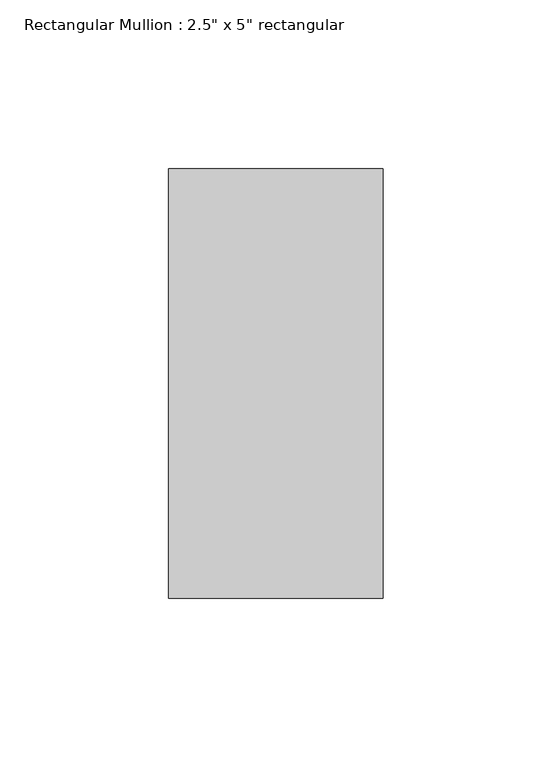
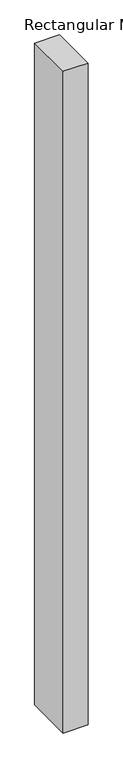
"""IFC4 building model written with IfcOpenShell, lengths in millimetres: member geometry."""

from ifc_helpers import new_model, si_unit, frame, origin, place, context, project, spatial, polyline, outline, extrude, source, transform, mapped, element, save


def member_f80a073c(model_context):
    return source(origin(), model_context, "Body", "SweptSolid", [
        extrude(outline(polyline([(0.0, 63.5), (0.0, -63.5), (-63.5, -63.5), (-63.5, 63.5), (0.0, 63.5)])), frame((0.0, 0.0, -1796.4671151), z_axis=(0.0, 0.0, 1.0), x_axis=(1.0, 0.0, 0.0)), (0.0, 0.0, 1.0), 1796.4671151),
    ])


if __name__ == "__main__":
    model = new_model("IFC4")
    model_context = context("Model", 3, world=origin())
    ifc_project = project(units=[si_unit("LENGTHUNIT", "METRE", prefix="MILLI")], contexts=[model_context])
    site = spatial("IfcSite", under=ifc_project)
    building = spatial("IfcBuilding", under=site)
    placement = place(None, origin())
    member_shape = member_f80a073c(model_context)
    element("IfcMember", 1, ObjectType="Rectangular Mullion : 2.5\" x 5\" rectangular", at=placement, inside=building, context=model_context, shape_type="MappedRepresentation", body=[
        mapped(member_shape, transform((0.0, 0.0, 0.0), x_axis=(1.0, 0.0, 0.0), y_axis=(0.0, 1.0, 0.0), z_axis=(0.0, 0.0, 1.0))),
    ])
    save(model, "model.ifc")

# Revit data of these elements
# Type "Rectangular Mullion : 2.5\" x 5\" rectangular"
#   built-in parameter 1007304 = 0.416667 (stored number, unit not read)
#   built-in parameter 1007301 = 0.104167 (stored number, unit not read)
#   built-in parameter 1007300 = 0.104167 (stored number, unit not read)
# Element 1 (IfcMember, "Rectangular Mullion : 2.5\" x 5\" rectangular")
#   Materials on its faces: "Aluminum"
# Materials
#   "Aluminum": class "Metal", colour RGB 247 247 247, transparency 0, Description = "Aluminum 6061", Cost = 0
